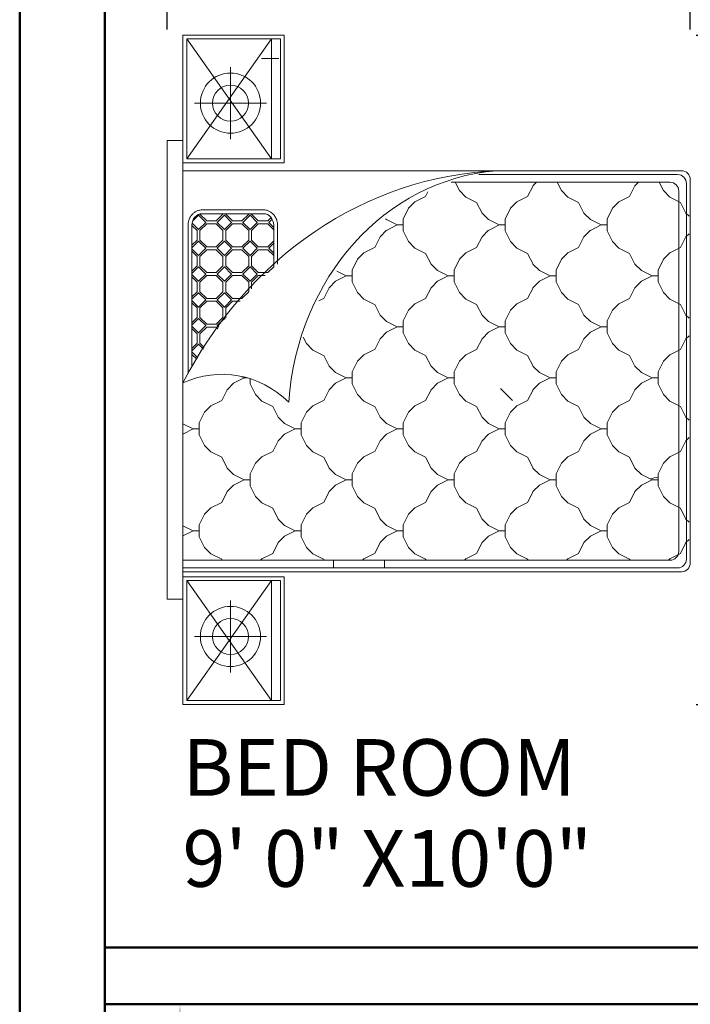
# Model space of a CAD drawing. Units: inches. Extents: x 2385 to 2740, y 1752 to 2305.
# Tile 8 of 15: x 2414 to 2485, y 2141 to 2245. Entities that reach past the tile are written whole.
import ezdxf

# ---------------------------------------------------------------- set-up
doc = ezdxf.new("R2010")
doc.units = ezdxf.units.IN
for name, color, linetype, lineweight in [('A-ANNO-DIMS', 2, 'Continuous', 18), ('A-AREA-IDEN', 7, 'Continuous', 25), ('A-FURN', 9, 'Continuous', 18), ('A-WALL', 7, 'Continuous', 50)]:
    doc.layers.add(name, color=color, linetype=linetype, lineweight=lineweight)
doc.styles.get("Standard").update_dxf_attribs({"font": 'arial.ttf'})
doc.dimstyles.new('Copy of ISO-25', dxfattribs={"dimtxt": 2.5, "dimasz": 2.5, "dimexe": 1.25, "dimexo": 0.625, "dimtad": 1, "dimdec": 1, "dimlunit": 4, "dimtxsty": 'Standard', "dimcen": 2.5, "dimadec": 0, "dimazin": 0, "dimtfac": 1, "dimtdec": 1, "dimtmove": 0, "dimatfit": 3, "dimfxl": 1, "dimarcsym": 0})

# ---------------------------------------------------------------- blocks, each defined once
blk = doc.blocks.new('A$C029D5C69')
for p, q in [((0.4164, 2.0693), (0.4164, 2.0066)), ((2.2315, 2.0693), (0.4164, 2.0693)), ((2.2315, 2.0066), (2.2315, 2.0693)), ((0, 1.606), (0, 2.0066)), ((0, 2.0066), (0.505, 2.0066)), ((0.0151, 1.6211), (0.0151, 1.9915)), ((0.0151, 1.9915), (0.4899, 1.9915)), ((0.4164, 2.0066), (2.2315, 2.0066)), ((0.4899, 1.9915), (0.4899, 1.6211)), ((0.505, 2.0066), (0.505, 1.606)), ((0.5252, 0.0351), (0.5252, 2.0066)), ((0.5403, 0.0502), (0.5403, 2.0066)), ((0.5706, 0.0805), (0.5706, 2.0066)), ((0.6869, 1.966), (0.6666, 2.0066)), ((0.7072, 2.0066), (0.6869, 1.966)), ((1.0902, 1.966), (1.0699, 2.0066)), ((1.1106, 2.0066), (1.0902, 1.966)), ((2.1114, 2.0087), (2.1114, 0.0351)), ((2.6479, 2.0066), (2.1429, 2.0066)), ((2.1429, 2.0066), (2.1429, 1.606)), ((2.6328, 1.9915), (2.158, 1.9915)), ((2.158, 1.9915), (2.158, 1.6211)), ((2.6328, 1.6211), (2.6328, 1.9915)), ((2.6479, 1.606), (2.6479, 2.0066)), ((0.2689, 1.9609), (0.2689, 1.6764)), ((0.6869, 1.9425), (0.6869, 1.966)), ((0.6869, 1.9425), (0.6869, 1.966)), ((1.0902, 1.9425), (1.0902, 1.966)), ((1.0902, 1.9425), (1.0902, 1.966)), ((1.8954, 1.9865), (1.3081, 1.9865)), ((1.8954, 1.9713), (1.3339, 1.9713)), ((1.3849, 1.9713), (1.3656, 1.952)), ((1.3945, 1.9713), (1.3714, 1.9483)), ((1.4249, 1.945), (1.3986, 1.9713)), ((1.4288, 1.9507), (1.4081, 1.9713)), ((1.4476, 1.9507), (1.4288, 1.9507)), ((1.4476, 1.9507), (1.4664, 1.9507)), ((1.487, 1.9713), (1.4664, 1.9507)), ((1.4966, 1.9713), (1.4703, 1.945)), ((1.527, 1.945), (1.5007, 1.9713)), ((1.5309, 1.9507), (1.5102, 1.9713)), ((1.5497, 1.9507), (1.5309, 1.9507)), ((1.5497, 1.9507), (1.5685, 1.9507)), ((1.5891, 1.9713), (1.5685, 1.9507)), ((1.5987, 1.9713), (1.5724, 1.945)), ((1.6291, 1.945), (1.6028, 1.9713)), ((1.633, 1.9507), (1.6123, 1.9713)), ((1.6518, 1.9507), (1.633, 1.9507)), ((1.6518, 1.9507), (1.6706, 1.9507)), ((1.6912, 1.9713), (1.6706, 1.9507)), ((1.7008, 1.9713), (1.6745, 1.945)), ((1.7312, 1.945), (1.7049, 1.9713)), ((1.7351, 1.9507), (1.7144, 1.9713)), ((1.7539, 1.9507), (1.7351, 1.9507)), ((1.7539, 1.9507), (1.7727, 1.9507)), ((1.7933, 1.9713), (1.7727, 1.9507)), ((1.8029, 1.9713), (1.7766, 1.945)), ((1.8333, 1.945), (1.807, 1.9713)), ((1.8372, 1.9507), (1.8165, 1.9713)), ((1.856, 1.9507), (1.8372, 1.9507)), ((1.856, 1.9507), (1.8748, 1.9507)), ((1.8954, 1.9713), (1.8748, 1.9507)), ((1.9043, 1.9707), (1.8787, 1.945)), ((1.9354, 1.945), (1.9114, 1.969)), ((2.379, 1.9609), (2.379, 1.6764)), ((0.621, 1.9213), (0.5955, 1.8958)), ((0.6634, 1.9425), (0.621, 1.9213)), ((0.6634, 1.9425), (0.621, 1.9213)), ((0.6869, 1.9425), (0.6634, 1.9425)), ((0.6869, 1.9425), (0.7104, 1.9425)), ((0.7528, 1.9213), (0.7104, 1.9425)), ((0.7528, 1.9213), (0.7104, 1.9425)), ((0.7783, 1.8958), (0.7528, 1.9213)), ((1.0243, 1.9213), (0.9988, 1.8958)), ((1.0668, 1.9425), (1.0244, 1.9213)), ((1.0668, 1.9425), (1.0244, 1.9213)), ((1.0902, 1.9425), (1.0668, 1.9425)), ((1.0902, 1.9425), (1.1137, 1.9425)), ((1.1561, 1.9213), (1.1137, 1.9425)), ((1.1561, 1.9213), (1.1137, 1.9425)), ((1.1816, 1.8958), (1.1561, 1.9213)), ((1.4249, 1.945), (1.4059, 1.926)), ((1.4288, 1.9394), (1.4116, 1.9222)), ((1.4288, 1.9393), (1.4476, 1.9393)), ((1.4664, 1.9393), (1.4476, 1.9393)), ((1.493, 1.9128), (1.4664, 1.9394)), ((1.4986, 1.9167), (1.4703, 1.945)), ((1.493, 1.8752), (1.493, 1.9128)), ((1.527, 1.945), (1.4986, 1.9167)), ((1.5309, 1.9394), (1.5043, 1.9128)), ((1.5043, 1.8752), (1.5043, 1.9128)), ((1.5309, 1.9393), (1.5497, 1.9393)), ((1.5685, 1.9393), (1.5497, 1.9393)), ((1.595, 1.9128), (1.5685, 1.9394)), ((1.6007, 1.9167), (1.5724, 1.945)), ((1.595, 1.8752), (1.595, 1.9128)), ((1.6291, 1.945), (1.6007, 1.9167)), ((1.633, 1.9394), (1.6064, 1.9128)), ((1.6064, 1.8752), (1.6064, 1.9128)), ((1.633, 1.9393), (1.6518, 1.9393)), ((1.6706, 1.9393), (1.6518, 1.9393)), ((1.6971, 1.9128), (1.6706, 1.9394)), ((1.7028, 1.9167), (1.6745, 1.945)), ((1.6971, 1.8752), (1.6971, 1.9128)), ((1.7312, 1.945), (1.7028, 1.9167)), ((1.7351, 1.9394), (1.7085, 1.9128)), ((1.7085, 1.8752), (1.7085, 1.9128)), ((1.7351, 1.9393), (1.7539, 1.9393)), ((1.7727, 1.9393), (1.7539, 1.9393)), ((1.7992, 1.9128), (1.7727, 1.9394)), ((1.8049, 1.9167), (1.7766, 1.945)), ((1.7992, 1.8752), (1.7992, 1.9128)), ((1.8333, 1.945), (1.8049, 1.9167)), ((1.8372, 1.9394), (1.8106, 1.9128)), ((1.8106, 1.8752), (1.8106, 1.9128)), ((1.8372, 1.9393), (1.856, 1.9393)), ((1.8748, 1.9393), (1.856, 1.9393)), ((1.9013, 1.9128), (1.8748, 1.9394)), ((1.907, 1.9167), (1.8787, 1.945)), ((1.9013, 1.8752), (1.9013, 1.9128)), ((1.9354, 1.945), (1.907, 1.9167)), ((1.9393, 1.9394), (1.9127, 1.9128)), ((1.9127, 1.8752), (1.9127, 1.9128)), ((1.9393, 1.9393), (1.9404, 1.9393)), ((1.9414, 1.688), (1.9414, 1.931)), ((1.9565, 1.688), (1.9565, 1.931)), ((0.5955, 1.8958), (0.5743, 1.8534)), ((0.7995, 1.8534), (0.7783, 1.8958)), ((0.9989, 1.8958), (0.9777, 1.8534)), ((1.2028, 1.8534), (1.1816, 1.8958)), ((1.493, 1.8752), (1.4867, 1.869)), ((1.4986, 1.8713), (1.4922, 1.8648)), ((1.527, 1.8429), (1.4986, 1.8713)), ((1.5309, 1.8486), (1.5043, 1.8752)), ((1.595, 1.8752), (1.5685, 1.8486)), ((1.6007, 1.8713), (1.5724, 1.8429)), ((1.6291, 1.8429), (1.6007, 1.8713)), ((1.633, 1.8486), (1.6064, 1.8752)), ((1.6971, 1.8752), (1.6706, 1.8486)), ((1.7028, 1.8713), (1.6745, 1.8429)), ((1.7312, 1.8429), (1.7028, 1.8713)), ((1.7351, 1.8486), (1.7085, 1.8752)), ((1.7992, 1.8752), (1.7727, 1.8486)), ((1.8049, 1.8713), (1.7766, 1.8429)), ((1.8333, 1.8429), (1.8049, 1.8713)), ((1.8372, 1.8486), (1.8106, 1.8752)), ((1.9013, 1.8752), (1.8748, 1.8486)), ((1.907, 1.8713), (1.8787, 1.8429)), ((1.9354, 1.8429), (1.907, 1.8713)), ((1.9393, 1.8486), (1.9127, 1.8752)), ((0.5743, 1.8534), (0.5706, 1.8515)), ((0.5743, 1.8534), (0.5706, 1.8515)), ((0.8419, 1.8322), (0.7995, 1.8534)), ((0.8419, 1.8322), (0.7995, 1.8534)), ((0.8674, 1.8067), (0.8419, 1.8322)), ((0.9352, 1.8322), (0.9097, 1.8067)), ((0.9777, 1.8534), (0.9353, 1.8322)), ((0.9777, 1.8534), (0.9353, 1.8322)), ((1.2452, 1.8322), (1.2028, 1.8534)), ((1.2452, 1.8322), (1.2028, 1.8534)), ((1.2707, 1.8067), (1.2452, 1.8322)), ((1.527, 1.8429), (1.5242, 1.8401)), ((1.5309, 1.8373), (1.5295, 1.8359)), ((1.5497, 1.8486), (1.5309, 1.8486)), ((1.5309, 1.8373), (1.5497, 1.8373)), ((1.5497, 1.8486), (1.5685, 1.8486)), ((1.5685, 1.8373), (1.5497, 1.8373)), ((1.595, 1.8107), (1.5685, 1.8373)), ((1.6007, 1.8146), (1.5724, 1.8429)), ((1.6291, 1.8429), (1.6007, 1.8146)), ((1.633, 1.8373), (1.6064, 1.8107)), ((1.6518, 1.8486), (1.633, 1.8486)), ((1.633, 1.8373), (1.6518, 1.8373)), ((1.6518, 1.8486), (1.6706, 1.8486)), ((1.6706, 1.8373), (1.6518, 1.8373)), ((1.6971, 1.8107), (1.6706, 1.8373)), ((1.7028, 1.8146), (1.6745, 1.8429)), ((1.7312, 1.8429), (1.7028, 1.8146)), ((1.7351, 1.8373), (1.7085, 1.8107)), ((1.7539, 1.8486), (1.7351, 1.8486)), ((1.7351, 1.8373), (1.7539, 1.8373)), ((1.7539, 1.8486), (1.7727, 1.8486)), ((1.7727, 1.8373), (1.7539, 1.8373)), ((1.7992, 1.8107), (1.7727, 1.8373)), ((1.8049, 1.8146), (1.7766, 1.8429)), ((1.8333, 1.8429), (1.8049, 1.8146)), ((1.8372, 1.8373), (1.8106, 1.8107)), ((1.856, 1.8486), (1.8372, 1.8486)), ((1.8372, 1.8373), (1.856, 1.8373)), ((1.856, 1.8486), (1.8748, 1.8486)), ((1.8748, 1.8373), (1.856, 1.8373)), ((1.9013, 1.8107), (1.8748, 1.8373)), ((1.907, 1.8146), (1.8787, 1.8429)), ((1.9354, 1.8429), (1.907, 1.8146)), ((1.9393, 1.8373), (1.9127, 1.8107)), ((1.9414, 1.8486), (1.9393, 1.8486)), ((1.9393, 1.8373), (1.9414, 1.8373)), ((0.1267, 1.8186), (0.4111, 1.8186)), ((0.8886, 1.7643), (0.8674, 1.8067)), ((0.9098, 1.8067), (0.8886, 1.7643)), ((1.2919, 1.7643), (1.2707, 1.8067)), ((1.595, 1.7806), (1.595, 1.8107)), ((1.6064, 1.7731), (1.6064, 1.8107)), ((1.6971, 1.7731), (1.6971, 1.8107)), ((1.7085, 1.7731), (1.7085, 1.8107)), ((1.7992, 1.7731), (1.7992, 1.8107)), ((1.8106, 1.7731), (1.8106, 1.8107)), ((1.9013, 1.7731), (1.9013, 1.8107)), ((1.9127, 1.7731), (1.9127, 1.8107)), ((2.2367, 1.8186), (2.5212, 1.8186)), ((0.8886, 1.7408), (0.8886, 1.7643)), ((1.2981, 1.7768), (1.2919, 1.7643)), ((1.2919, 1.7519), (1.2919, 1.7643)), ((1.633, 1.7465), (1.6064, 1.7731)), ((1.6971, 1.7731), (1.6706, 1.7465)), ((1.7028, 1.7692), (1.6745, 1.7408)), ((1.7312, 1.7408), (1.7028, 1.7692)), ((1.7351, 1.7465), (1.7085, 1.7731)), ((1.7992, 1.7731), (1.7727, 1.7465)), ((1.8049, 1.7692), (1.7766, 1.7408)), ((1.8333, 1.7408), (1.8049, 1.7692)), ((1.8372, 1.7465), (1.8106, 1.7731)), ((1.9013, 1.7731), (1.8748, 1.7465)), ((1.907, 1.7692), (1.8787, 1.7408)), ((1.9354, 1.7408), (1.907, 1.7692)), ((1.9393, 1.7465), (1.9127, 1.7731)), ((0.8227, 1.7196), (0.7972, 1.6941)), ((0.8651, 1.7408), (0.8227, 1.7196)), ((0.8651, 1.7408), (0.8227, 1.7196)), ((0.912, 1.7408), (0.8651, 1.7408)), ((0.9544, 1.7196), (0.912, 1.7408)), ((0.9544, 1.7196), (0.912, 1.7408)), ((0.98, 1.6941), (0.9545, 1.7196)), ((1.226, 1.7196), (1.2005, 1.6941)), ((1.2684, 1.7408), (1.226, 1.7196)), ((1.2684, 1.7408), (1.226, 1.7196)), ((1.2885, 1.7408), (1.2684, 1.7408)), ((1.6518, 1.7465), (1.633, 1.7465)), ((1.6443, 1.7352), (1.6518, 1.7352)), ((1.6518, 1.7465), (1.6706, 1.7465)), ((1.6706, 1.7352), (1.6518, 1.7352)), ((1.6971, 1.7086), (1.6706, 1.7352)), ((1.7028, 1.7125), (1.6745, 1.7408)), ((1.7312, 1.7408), (1.7028, 1.7125)), ((1.7351, 1.7352), (1.7085, 1.7086)), ((1.7539, 1.7465), (1.7351, 1.7465)), ((1.7351, 1.7352), (1.7539, 1.7352)), ((1.7539, 1.7465), (1.7727, 1.7465)), ((1.7727, 1.7352), (1.7539, 1.7352)), ((1.7992, 1.7086), (1.7727, 1.7352)), ((1.8049, 1.7125), (1.7766, 1.7408)), ((1.8333, 1.7408), (1.8049, 1.7125)), ((1.8372, 1.7352), (1.8106, 1.7086)), ((1.856, 1.7465), (1.8372, 1.7465)), ((1.8372, 1.7352), (1.856, 1.7352)), ((1.856, 1.7465), (1.8748, 1.7465)), ((1.8748, 1.7352), (1.856, 1.7352)), ((1.9013, 1.7086), (1.8748, 1.7352)), ((1.907, 1.7125), (1.8787, 1.7408)), ((1.9354, 1.7408), (1.907, 1.7125)), ((1.9393, 1.7352), (1.9127, 1.7086)), ((1.9414, 1.7465), (1.9393, 1.7465)), ((1.9393, 1.7352), (1.9414, 1.7352)), ((0.5766, 1.6941), (0.5706, 1.7002)), ((0.5978, 1.6517), (0.5766, 1.6941)), ((0.7972, 1.6941), (0.776, 1.6517)), ((1.0011, 1.6517), (0.9799, 1.6941)), ((1.2005, 1.6941), (1.1793, 1.6517)), ((1.6971, 1.682), (1.6971, 1.7086)), ((1.7085, 1.671), (1.7085, 1.7086)), ((1.7992, 1.671), (1.7992, 1.7086)), ((1.8106, 1.671), (1.8106, 1.7086)), ((1.9013, 1.671), (1.9013, 1.7086)), ((1.9127, 1.671), (1.9127, 1.7086)), ((2.5551, 1.6275), (2.5551, 1.696)), ((0.6402, 1.6305), (0.5978, 1.6517)), ((0.6402, 1.6305), (0.5978, 1.6517)), ((0.776, 1.6517), (0.7336, 1.6305)), ((0.776, 1.6517), (0.7336, 1.6305)), ((1.0435, 1.6305), (1.0011, 1.6517)), ((1.0435, 1.6305), (1.0011, 1.6517)), ((1.1793, 1.6517), (1.1369, 1.6305)), ((1.1793, 1.6517), (1.1369, 1.6305)), ((1.7318, 1.6477), (1.7085, 1.671)), ((1.8961, 1.6477), (1.7289, 1.6477)), ((1.7992, 1.671), (1.7759, 1.6477)), ((1.8049, 1.6671), (1.7855, 1.6477)), ((1.8244, 1.6477), (1.8049, 1.6671)), ((1.8339, 1.6477), (1.8106, 1.671)), ((1.9013, 1.671), (1.878, 1.6477)), ((1.907, 1.6671), (1.8876, 1.6477)), ((1.9202, 1.6539), (1.907, 1.6671)), ((1.926, 1.6577), (1.9127, 1.671)), ((0.505, 1.606), (0, 1.606)), ((0.4899, 1.6211), (0.0151, 1.6211)), ((0.6657, 1.605), (0.6402, 1.6305)), ((0.6869, 1.5626), (0.6657, 1.605)), ((0.7081, 1.605), (0.6869, 1.5626)), ((0.7336, 1.6305), (0.7081, 1.605)), ((1.0691, 1.605), (1.0436, 1.6305)), ((1.0902, 1.5626), (1.069, 1.605)), ((1.1114, 1.605), (1.0902, 1.5626)), ((1.1369, 1.6305), (1.1114, 1.605)), ((1.8961, 1.6325), (1.7422, 1.6325)), ((2.1429, 1.606), (2.6479, 1.606)), ((2.158, 1.6211), (2.6328, 1.6211)), ((0.6869, 1.5392), (0.6869, 1.5626)), ((0.6869, 1.5392), (0.6869, 1.5626)), ((1.0902, 1.5392), (1.0902, 1.5626)), ((1.0902, 1.5392), (1.0902, 1.5626)), ((0.6634, 1.5391), (0.621, 1.5179)), ((0.6634, 1.5391), (0.621, 1.5179)), ((0.6869, 1.5392), (0.6634, 1.5392)), ((0.6869, 1.5392), (0.7104, 1.5392)), ((0.7528, 1.5179), (0.7104, 1.5391)), ((0.7528, 1.5179), (0.7104, 1.5391)), ((1.0668, 1.5391), (1.0244, 1.5179)), ((1.0668, 1.5391), (1.0244, 1.5179)), ((1.0902, 1.5392), (1.0668, 1.5392)), ((1.0902, 1.5392), (1.1137, 1.5392)), ((1.1561, 1.5179), (1.1137, 1.5391)), ((1.1561, 1.5179), (1.1137, 1.5391)), ((1.4534, 1.5308), (1.4277, 1.5179)), ((1.4534, 1.5308), (1.4277, 1.5179)), ((0.5955, 1.4925), (0.5743, 1.4501)), ((0.621, 1.5179), (0.5955, 1.4924)), ((0.7783, 1.4924), (0.7528, 1.5179)), ((0.7995, 1.4501), (0.7783, 1.4925)), ((0.9989, 1.4925), (0.9777, 1.4501)), ((1.0243, 1.5179), (0.9988, 1.4924)), ((1.1816, 1.4924), (1.1561, 1.5179)), ((1.2028, 1.4501), (1.1816, 1.4925)), ((1.4022, 1.4925), (1.381, 1.4501)), ((1.4277, 1.5179), (1.4022, 1.4924)), ((0.5743, 1.45), (0.5706, 1.4481)), ((0.5743, 1.45), (0.5706, 1.4481)), ((0.8419, 1.4288), (0.7995, 1.45)), ((0.8419, 1.4288), (0.7995, 1.45)), ((0.9777, 1.45), (0.9353, 1.4288)), ((0.9777, 1.45), (0.9353, 1.4288)), ((1.2452, 1.4288), (1.2028, 1.45)), ((1.2452, 1.4288), (1.2028, 1.45)), ((1.381, 1.45), (1.3386, 1.4288)), ((1.381, 1.45), (1.3386, 1.4288)), ((1.6062, 1.4501), (1.5966, 1.4692)), ((1.6486, 1.4288), (1.6062, 1.45)), ((1.6486, 1.4288), (1.6062, 1.45)), ((0.5403, 1.4117), (0.5706, 1.4117)), ((0.8674, 1.4033), (0.8419, 1.4288)), ((0.8886, 1.361), (0.8674, 1.4034)), ((0.9098, 1.4034), (0.8886, 1.361)), ((0.9352, 1.4288), (0.9097, 1.4033)), ((1.2707, 1.4033), (1.2452, 1.4288)), ((1.2919, 1.361), (1.2707, 1.4034)), ((1.3131, 1.4034), (1.2919, 1.361)), ((1.3386, 1.4288), (1.3131, 1.4033)), ((1.6741, 1.4033), (1.6486, 1.4288)), ((1.6953, 1.361), (1.6741, 1.4034)), ((1.714, 1.3984), (1.6953, 1.361)), ((0.8651, 1.3374), (0.8227, 1.3162)), ((0.8651, 1.3374), (0.8227, 1.3162)), ((0.912, 1.3375), (0.8651, 1.3375)), ((0.8886, 1.3375), (0.8886, 1.3609)), ((0.9544, 1.3162), (0.912, 1.3374)), ((0.9544, 1.3162), (0.912, 1.3374)), ((1.2684, 1.3374), (1.226, 1.3162)), ((1.2684, 1.3374), (1.226, 1.3162)), ((1.3154, 1.3375), (1.2684, 1.3375)), ((1.2919, 1.3375), (1.2919, 1.3609)), ((1.3578, 1.3162), (1.3154, 1.3374)), ((1.3578, 1.3162), (1.3154, 1.3374)), ((1.6718, 1.3374), (1.6294, 1.3162)), ((1.6718, 1.3374), (1.6294, 1.3162)), ((1.7187, 1.3375), (1.6718, 1.3375)), ((1.6953, 1.3375), (1.6953, 1.3609)), ((1.7611, 1.3162), (1.7187, 1.3374)), ((1.7611, 1.3162), (1.7187, 1.3374)), ((0.5766, 1.2908), (0.5706, 1.2968)), ((0.5978, 1.2484), (0.5766, 1.2908)), ((0.7972, 1.2908), (0.776, 1.2484)), ((0.8227, 1.3163), (0.7972, 1.2908)), ((0.98, 1.2908), (0.9545, 1.3163)), ((1.0011, 1.2484), (0.9799, 1.2908)), ((1.2005, 1.2908), (1.1793, 1.2484)), ((1.226, 1.3163), (1.2005, 1.2908)), ((1.3833, 1.2908), (1.3578, 1.3163)), ((1.4045, 1.2484), (1.3833, 1.2908)), ((1.6039, 1.2908), (1.5827, 1.2484)), ((1.6294, 1.3163), (1.6039, 1.2908)), ((1.7867, 1.2908), (1.7611, 1.3163)), ((1.8078, 1.2484), (1.7866, 1.2908)), ((0.6402, 1.2271), (0.5978, 1.2483)), ((0.6402, 1.2271), (0.5978, 1.2483)), ((0.776, 1.2483), (0.7336, 1.2271)), ((0.776, 1.2483), (0.7336, 1.2271)), ((1.0435, 1.2271), (1.0011, 1.2483)), ((1.0435, 1.2271), (1.0011, 1.2483)), ((1.1793, 1.2483), (1.1369, 1.2271)), ((1.1793, 1.2483), (1.1369, 1.2271)), ((1.4469, 1.2271), (1.4045, 1.2483)), ((1.4469, 1.2271), (1.4045, 1.2483)), ((1.5827, 1.2483), (1.5403, 1.2271)), ((1.5827, 1.2483), (1.5403, 1.2271)), ((1.8502, 1.2271), (1.8078, 1.2483)), ((1.8502, 1.2271), (1.8078, 1.2483)), ((0.5403, 1.21), (0.5706, 1.21)), ((0.6657, 1.2017), (0.6402, 1.2272)), ((0.7336, 1.2272), (0.7081, 1.2017)), ((1.0691, 1.2017), (1.0436, 1.2272)), ((1.1369, 1.2272), (1.1114, 1.2017)), ((1.4724, 1.2017), (1.4469, 1.2272)), ((1.5403, 1.2272), (1.5148, 1.2017)), ((1.8758, 1.2017), (1.8503, 1.2272)), ((0.6869, 1.1593), (0.6657, 1.2017)), ((0.7081, 1.2017), (0.6869, 1.1593)), ((1.0902, 1.1593), (1.069, 1.2017)), ((1.1114, 1.2017), (1.0902, 1.1593)), ((1.4936, 1.1593), (1.4724, 1.2017)), ((1.5148, 1.2017), (1.4936, 1.1593)), ((1.8969, 1.1593), (1.8757, 1.2017)), ((1.9181, 1.2017), (1.8969, 1.1593)), ((1.9215, 1.2051), (1.9181, 1.2017)), ((0.6634, 1.1358), (0.621, 1.1146)), ((0.6634, 1.1358), (0.621, 1.1146)), ((0.6869, 1.1358), (0.6634, 1.1358)), ((0.6869, 1.1358), (0.6869, 1.1593)), ((0.6869, 1.1358), (0.6869, 1.1593)), ((0.6869, 1.1358), (0.7104, 1.1358)), ((0.7528, 1.1146), (0.7104, 1.1358)), ((0.7528, 1.1146), (0.7104, 1.1358)), ((1.0668, 1.1358), (1.0244, 1.1146)), ((1.0668, 1.1358), (1.0244, 1.1146)), ((1.0902, 1.1358), (1.0668, 1.1358)), ((1.0902, 1.1358), (1.0902, 1.1593)), ((1.0902, 1.1358), (1.0902, 1.1593)), ((1.0902, 1.1358), (1.1137, 1.1358)), ((1.1561, 1.1146), (1.1137, 1.1358)), ((1.1561, 1.1146), (1.1137, 1.1358)), ((1.4701, 1.1358), (1.4277, 1.1146)), ((1.4701, 1.1358), (1.4277, 1.1146)), ((1.4936, 1.1358), (1.4701, 1.1358)), ((1.4936, 1.1358), (1.4936, 1.1593)), ((1.4936, 1.1358), (1.4936, 1.1593)), ((1.4936, 1.1358), (1.5171, 1.1358)), ((1.5595, 1.1146), (1.5171, 1.1358)), ((1.5595, 1.1146), (1.5171, 1.1358)), ((1.8735, 1.1358), (1.8311, 1.1146)), ((1.8735, 1.1358), (1.8311, 1.1146)), ((1.8969, 1.1358), (1.8735, 1.1358)), ((1.8969, 1.1358), (1.8969, 1.1593)), ((1.8969, 1.1358), (1.8969, 1.1593)), ((1.8969, 1.1358), (1.9204, 1.1358)), ((1.9628, 1.1146), (1.9204, 1.1358)), ((1.9628, 1.1146), (1.9204, 1.1358)), ((0.621, 1.1146), (0.5955, 1.0891)), ((0.7783, 1.0891), (0.7528, 1.1146)), ((1.0243, 1.1146), (0.9988, 1.0891)), ((1.1816, 1.0891), (1.1561, 1.1146)), ((1.4277, 1.1146), (1.4022, 1.0891)), ((1.585, 1.0891), (1.5595, 1.1146)), ((1.831, 1.1146), (1.8055, 1.0891)), ((1.9883, 1.0891), (1.9628, 1.1146)), ((0.5955, 1.0891), (0.5743, 1.0467)), ((0.7995, 1.0467), (0.7783, 1.0891)), ((0.9989, 1.0891), (0.9777, 1.0467)), ((1.2028, 1.0467), (1.1816, 1.0891)), ((1.4022, 1.0891), (1.381, 1.0467)), ((1.6062, 1.0467), (1.585, 1.0891)), ((1.8056, 1.0891), (1.7844, 1.0467)), ((2.0095, 1.0467), (1.9883, 1.0891)), ((0.5743, 1.0467), (0.5706, 1.0448)), ((0.5743, 1.0467), (0.5706, 1.0448)), ((0.8419, 1.0255), (0.7995, 1.0467)), ((0.8419, 1.0255), (0.7995, 1.0467)), ((0.8674, 1), (0.8419, 1.0255)), ((0.9352, 1.0255), (0.9097, 1)), ((0.9777, 1.0467), (0.9353, 1.0255)), ((0.9777, 1.0467), (0.9353, 1.0255)), ((1.2452, 1.0255), (1.2028, 1.0467)), ((1.2452, 1.0255), (1.2028, 1.0467)), ((1.2707, 1), (1.2452, 1.0255)), ((1.3386, 1.0255), (1.3131, 1)), ((1.381, 1.0467), (1.3386, 1.0255)), ((1.381, 1.0467), (1.3386, 1.0255)), ((1.6486, 1.0255), (1.6062, 1.0467)), ((1.6486, 1.0255), (1.6062, 1.0467)), ((1.6741, 1), (1.6486, 1.0255)), ((1.7419, 1.0255), (1.7164, 1)), ((1.7844, 1.0467), (1.742, 1.0255)), ((1.7844, 1.0467), (1.742, 1.0255)), ((2.0276, 1.0376), (2.0095, 1.0467)), ((2.0276, 1.0376), (2.0095, 1.0467)), ((0.8886, 0.9576), (0.8674, 1)), ((0.9098, 1), (0.8886, 0.9576)), ((1.2919, 0.9576), (1.2707, 1)), ((1.3131, 1), (1.2919, 0.9576)), ((1.6953, 0.9576), (1.6741, 1)), ((1.7165, 1), (1.6953, 0.9576)), ((0.8886, 0.9341), (0.8886, 0.9576)), ((1.2919, 0.9341), (1.2919, 0.9576)), ((1.6953, 0.9341), (1.6953, 0.9576)), ((2.066, 0.9457), (2.066, 0.0805)), ((0.8227, 0.9129), (0.7972, 0.8874)), ((0.8651, 0.9341), (0.8227, 0.9129)), ((0.8651, 0.9341), (0.8227, 0.9129)), ((0.912, 0.9341), (0.8651, 0.9341)), ((0.9544, 0.9129), (0.912, 0.9341)), ((0.9544, 0.9129), (0.912, 0.9341)), ((0.98, 0.8874), (0.9545, 0.9129)), ((1.226, 0.9129), (1.2005, 0.8874)), ((1.2684, 0.9341), (1.226, 0.9129)), ((1.2684, 0.9341), (1.226, 0.9129)), ((1.3154, 0.9341), (1.2684, 0.9341)), ((1.3578, 0.9129), (1.3154, 0.9341)), ((1.3578, 0.9129), (1.3154, 0.9341)), ((1.3833, 0.8874), (1.3578, 0.9129)), ((1.6294, 0.9129), (1.6039, 0.8874)), ((1.6718, 0.9341), (1.6294, 0.9129)), ((1.6718, 0.9341), (1.6294, 0.9129)), ((1.7187, 0.9341), (1.6718, 0.9341)), ((1.7611, 0.9129), (1.7187, 0.9341)), ((1.7611, 0.9129), (1.7187, 0.9341)), ((1.7867, 0.8874), (1.7611, 0.9129)), ((2.0327, 0.9129), (2.0072, 0.8874)), ((2.066, 0.9295), (2.0327, 0.9129)), ((2.066, 0.9295), (2.0327, 0.9129)), ((0.5766, 0.8874), (0.5706, 0.8935)), ((0.5978, 0.845), (0.5766, 0.8874)), ((0.7972, 0.8874), (0.776, 0.845)), ((1.0011, 0.845), (0.9799, 0.8874)), ((1.2005, 0.8874), (1.1793, 0.845)), ((1.4045, 0.845), (1.3833, 0.8874)), ((1.6039, 0.8874), (1.5827, 0.845)), ((1.8078, 0.845), (1.7866, 0.8874)), ((2.0072, 0.8874), (1.986, 0.845)), ((0.6402, 0.8238), (0.5978, 0.845)), ((0.6402, 0.8238), (0.5978, 0.845)), ((0.6657, 0.7983), (0.6402, 0.8238)), ((0.7336, 0.8238), (0.7081, 0.7983)), ((0.776, 0.845), (0.7336, 0.8238)), ((0.776, 0.845), (0.7336, 0.8238)), ((1.0435, 0.8238), (1.0011, 0.845)), ((1.0435, 0.8238), (1.0011, 0.845)), ((1.0691, 0.7983), (1.0436, 0.8238)), ((1.1369, 0.8238), (1.1114, 0.7983)), ((1.1793, 0.845), (1.1369, 0.8238)), ((1.1793, 0.845), (1.1369, 0.8238)), ((1.4469, 0.8238), (1.4045, 0.845)), ((1.4469, 0.8238), (1.4045, 0.845)), ((1.4724, 0.7983), (1.4469, 0.8238)), ((1.5403, 0.8238), (1.5148, 0.7983)), ((1.5827, 0.845), (1.5403, 0.8238)), ((1.5827, 0.845), (1.5403, 0.8238)), ((1.8502, 0.8238), (1.8078, 0.845)), ((1.8502, 0.8238), (1.8078, 0.845)), ((1.8758, 0.7983), (1.8503, 0.8238)), ((1.9436, 0.8238), (1.9181, 0.7983)), ((1.986, 0.845), (1.9436, 0.8238)), ((1.986, 0.845), (1.9436, 0.8238)), ((2.0962, 0.8369), (2.0962, 0.0502)), ((0.6869, 0.7559), (0.6657, 0.7983)), ((0.7081, 0.7983), (0.6869, 0.7559)), ((1.0902, 0.7559), (1.069, 0.7983)), ((1.1114, 0.7983), (1.0902, 0.7559)), ((1.4936, 0.7559), (1.4724, 0.7983)), ((1.5148, 0.7983), (1.4936, 0.7559)), ((1.8969, 0.7559), (1.8757, 0.7983)), ((1.9181, 0.7983), (1.8969, 0.7559)), ((0.6869, 0.7325), (0.6869, 0.7559)), ((0.6869, 0.7325), (0.6869, 0.7559)), ((1.0902, 0.7325), (1.0902, 0.7559)), ((1.0902, 0.7325), (1.0902, 0.7559)), ((1.2024, 0.7028), (1.2503, 0.7507)), ((1.4936, 0.7325), (1.4936, 0.7559)), ((1.4936, 0.7325), (1.4936, 0.7559)), ((1.8969, 0.7325), (1.8969, 0.7559)), ((1.8969, 0.7325), (1.8969, 0.7559)), ((0.621, 0.7113), (0.5955, 0.6858)), ((0.6634, 0.7324), (0.621, 0.7112)), ((0.6634, 0.7324), (0.621, 0.7112)), ((0.6869, 0.7325), (0.6634, 0.7325)), ((0.6869, 0.7325), (0.7104, 0.7325)), ((0.7528, 0.7112), (0.7104, 0.7324)), ((0.7528, 0.7112), (0.7104, 0.7324)), ((0.7783, 0.6858), (0.7528, 0.7113)), ((1.0243, 0.7113), (0.9988, 0.6858)), ((1.0668, 0.7324), (1.0244, 0.7112)), ((1.0668, 0.7324), (1.0244, 0.7112)), ((1.0902, 0.7325), (1.0668, 0.7325)), ((1.0902, 0.7325), (1.1137, 0.7325)), ((1.1561, 0.7112), (1.1137, 0.7324)), ((1.1561, 0.7112), (1.1137, 0.7324)), ((1.1816, 0.6858), (1.1561, 0.7113)), ((1.4277, 0.7113), (1.4022, 0.6858)), ((1.4701, 0.7324), (1.4277, 0.7112)), ((1.4701, 0.7324), (1.4277, 0.7112)), ((1.4936, 0.7325), (1.4701, 0.7325)), ((1.4936, 0.7325), (1.5171, 0.7325)), ((1.5595, 0.7112), (1.5171, 0.7324)), ((1.5595, 0.7112), (1.5171, 0.7324)), ((1.585, 0.6858), (1.5595, 0.7113)), ((1.831, 0.7113), (1.8055, 0.6858)), ((1.8735, 0.7324), (1.8311, 0.7112)), ((1.8735, 0.7324), (1.8311, 0.7112)), ((1.8969, 0.7325), (1.8735, 0.7325)), ((1.8969, 0.7325), (1.9204, 0.7325)), ((1.9628, 0.7112), (1.9204, 0.7324)), ((1.9628, 0.7112), (1.9204, 0.7324)), ((1.9883, 0.6858), (1.9628, 0.7113)), ((0.5955, 0.6858), (0.5743, 0.6434)), ((0.7995, 0.6434), (0.7783, 0.6858)), ((0.9989, 0.6858), (0.9777, 0.6434)), ((1.2028, 0.6434), (1.1816, 0.6858)), ((1.4022, 0.6858), (1.381, 0.6434)), ((1.6062, 0.6434), (1.585, 0.6858)), ((1.8056, 0.6858), (1.7844, 0.6434)), ((2.0095, 0.6434), (1.9883, 0.6858)), ((0.5743, 0.6433), (0.5706, 0.6414)), ((0.5743, 0.6433), (0.5706, 0.6414)), ((0.8419, 0.6221), (0.7995, 0.6433)), ((0.8419, 0.6221), (0.7995, 0.6433)), ((0.9777, 0.6433), (0.9353, 0.6221)), ((0.9777, 0.6433), (0.9353, 0.6221)), ((1.2452, 0.6221), (1.2028, 0.6433)), ((1.2452, 0.6221), (1.2028, 0.6433)), ((1.381, 0.6433), (1.3386, 0.6221)), ((1.381, 0.6433), (1.3386, 0.6221)), ((1.6486, 0.6221), (1.6062, 0.6433)), ((1.6486, 0.6221), (1.6062, 0.6433)), ((1.7844, 0.6433), (1.742, 0.6221)), ((1.7844, 0.6433), (1.742, 0.6221)), ((2.0519, 0.6221), (2.0095, 0.6433)), ((2.0519, 0.6221), (2.0095, 0.6433)), ((0.8674, 0.5967), (0.8419, 0.6222)), ((0.8886, 0.5543), (0.8674, 0.5967)), ((0.9098, 0.5967), (0.8886, 0.5543)), ((0.9352, 0.6222), (0.9097, 0.5967)), ((1.2707, 0.5967), (1.2452, 0.6222)), ((1.2919, 0.5543), (1.2707, 0.5967)), ((1.3131, 0.5967), (1.2919, 0.5543)), ((1.3386, 0.6222), (1.3131, 0.5967)), ((1.6741, 0.5967), (1.6486, 0.6222)), ((1.6953, 0.5543), (1.6741, 0.5967)), ((1.7165, 0.5967), (1.6953, 0.5543)), ((1.7419, 0.6222), (1.7164, 0.5967)), ((2.066, 0.6081), (2.0519, 0.6222)), ((0.8886, 0.5308), (0.8886, 0.5543)), ((1.2919, 0.5308), (1.2919, 0.5543)), ((1.6953, 0.5308), (1.6953, 0.5543)), ((0.8227, 0.5096), (0.7972, 0.4841)), ((0.8651, 0.5308), (0.8227, 0.5096)), ((0.8651, 0.5308), (0.8227, 0.5096)), ((0.912, 0.5308), (0.8651, 0.5308)), ((0.9544, 0.5096), (0.912, 0.5308)), ((0.9544, 0.5096), (0.912, 0.5308)), ((0.98, 0.4841), (0.9545, 0.5096)), ((1.226, 0.5096), (1.2005, 0.4841)), ((1.2684, 0.5308), (1.226, 0.5096)), ((1.2684, 0.5308), (1.226, 0.5096)), ((1.3154, 0.5308), (1.2684, 0.5308)), ((1.3578, 0.5096), (1.3154, 0.5308)), ((1.3578, 0.5096), (1.3154, 0.5308)), ((1.3833, 0.4841), (1.3578, 0.5096)), ((1.6294, 0.5096), (1.6039, 0.4841)), ((1.6718, 0.5308), (1.6294, 0.5096)), ((1.6718, 0.5308), (1.6294, 0.5096)), ((1.7187, 0.5308), (1.6718, 0.5308)), ((1.7611, 0.5096), (1.7187, 0.5308)), ((1.7611, 0.5096), (1.7187, 0.5308)), ((1.7867, 0.4841), (1.7611, 0.5096)), ((2.0327, 0.5096), (2.0072, 0.4841)), ((2.066, 0.5262), (2.0327, 0.5096)), ((2.066, 0.5262), (2.0327, 0.5096)), ((0.5766, 0.4841), (0.5706, 0.4901)), ((0.5978, 0.4417), (0.5766, 0.4841)), ((0.7972, 0.4841), (0.776, 0.4417)), ((1.0011, 0.4417), (0.9799, 0.4841)), ((1.2005, 0.4841), (1.1793, 0.4417)), ((1.4045, 0.4417), (1.3833, 0.4841)), ((1.6039, 0.4841), (1.5827, 0.4417)), ((1.8078, 0.4417), (1.7866, 0.4841)), ((2.0072, 0.4841), (1.986, 0.4417)), ((0.6402, 0.4205), (0.5978, 0.4417)), ((0.6402, 0.4205), (0.5978, 0.4417)), ((0.776, 0.4417), (0.7336, 0.4205)), ((0.776, 0.4417), (0.7336, 0.4205)), ((1.0435, 0.4205), (1.0011, 0.4417)), ((1.0435, 0.4205), (1.0011, 0.4417)), ((1.1793, 0.4417), (1.1369, 0.4205)), ((1.1793, 0.4417), (1.1369, 0.4205)), ((1.4469, 0.4205), (1.4045, 0.4417)), ((1.4469, 0.4205), (1.4045, 0.4417)), ((1.5827, 0.4417), (1.5403, 0.4205)), ((1.5827, 0.4417), (1.5403, 0.4205)), ((1.8502, 0.4205), (1.8078, 0.4417)), ((1.8502, 0.4205), (1.8078, 0.4417)), ((1.986, 0.4417), (1.9436, 0.4205)), ((1.986, 0.4417), (1.9436, 0.4205)), ((0.6657, 0.395), (0.6402, 0.4205)), ((0.6869, 0.3526), (0.6657, 0.395)), ((0.7081, 0.395), (0.6869, 0.3526)), ((0.7336, 0.4205), (0.7081, 0.395)), ((1.0691, 0.395), (1.0436, 0.4205)), ((1.0902, 0.3526), (1.069, 0.395)), ((1.1114, 0.395), (1.0902, 0.3526)), ((1.1369, 0.4205), (1.1114, 0.395)), ((1.4724, 0.395), (1.4469, 0.4205)), ((1.4936, 0.3526), (1.4724, 0.395)), ((1.5148, 0.395), (1.4936, 0.3526)), ((1.5403, 0.4205), (1.5148, 0.395)), ((1.8758, 0.395), (1.8503, 0.4205)), ((1.8969, 0.3526), (1.8757, 0.395)), ((1.9181, 0.395), (1.8969, 0.3526)), ((1.9436, 0.4205), (1.9181, 0.395)), ((0.6869, 0.3291), (0.6869, 0.3526)), ((0.6869, 0.3291), (0.6869, 0.3526)), ((1.0902, 0.3291), (1.0902, 0.3526)), ((1.0902, 0.3291), (1.0902, 0.3526)), ((1.4936, 0.3291), (1.4936, 0.3526)), ((1.4936, 0.3291), (1.4936, 0.3526)), ((1.8969, 0.3291), (1.8969, 0.3526)), ((1.8969, 0.3291), (1.8969, 0.3526)), ((0.6634, 0.3291), (0.621, 0.3079)), ((0.6634, 0.3291), (0.621, 0.3079)), ((0.6869, 0.3291), (0.6634, 0.3291)), ((0.6869, 0.3291), (0.7104, 0.3291)), ((0.7528, 0.3079), (0.7104, 0.3291)), ((0.7528, 0.3079), (0.7104, 0.3291)), ((1.0668, 0.3291), (1.0244, 0.3079)), ((1.0668, 0.3291), (1.0244, 0.3079)), ((1.0902, 0.3291), (1.0668, 0.3291)), ((1.0902, 0.3291), (1.1137, 0.3291)), ((1.1561, 0.3079), (1.1137, 0.3291)), ((1.1561, 0.3079), (1.1137, 0.3291)), ((1.4701, 0.3291), (1.4277, 0.3079)), ((1.4701, 0.3291), (1.4277, 0.3079)), ((1.4936, 0.3291), (1.4701, 0.3291)), ((1.4936, 0.3291), (1.5171, 0.3291)), ((1.5595, 0.3079), (1.5171, 0.3291)), ((1.5595, 0.3079), (1.5171, 0.3291)), ((1.8735, 0.3291), (1.8311, 0.3079)), ((1.8735, 0.3291), (1.8311, 0.3079)), ((1.8969, 0.3291), (1.8735, 0.3291)), ((1.8969, 0.3291), (1.9204, 0.3291)), ((1.9628, 0.3079), (1.9204, 0.3291)), ((1.9628, 0.3079), (1.9204, 0.3291)), ((0.5955, 0.2824), (0.5743, 0.24)), ((0.621, 0.3079), (0.5955, 0.2824)), ((0.7783, 0.2824), (0.7528, 0.3079)), ((0.7995, 0.24), (0.7783, 0.2824)), ((0.9989, 0.2824), (0.9777, 0.24)), ((1.0243, 0.3079), (0.9988, 0.2824)), ((1.1816, 0.2824), (1.1561, 0.3079)), ((1.2028, 0.24), (1.1816, 0.2824)), ((1.4022, 0.2824), (1.381, 0.24)), ((1.4277, 0.3079), (1.4022, 0.2824)), ((1.585, 0.2824), (1.5595, 0.3079)), ((1.6062, 0.24), (1.585, 0.2824)), ((1.8056, 0.2824), (1.7844, 0.24)), ((1.831, 0.3079), (1.8055, 0.2824)), ((1.9883, 0.2824), (1.9628, 0.3079)), ((2.0095, 0.24), (1.9883, 0.2824)), ((0.5743, 0.24), (0.5706, 0.2381)), ((0.5743, 0.24), (0.5706, 0.2381)), ((0.8419, 0.2188), (0.7995, 0.24)), ((0.8419, 0.2188), (0.7995, 0.24)), ((0.9777, 0.24), (0.9353, 0.2188)), ((0.9777, 0.24), (0.9353, 0.2188)), ((1.2452, 0.2188), (1.2028, 0.24)), ((1.2452, 0.2188), (1.2028, 0.24)), ((1.381, 0.24), (1.3386, 0.2188)), ((1.381, 0.24), (1.3386, 0.2188)), ((1.6486, 0.2188), (1.6062, 0.24)), ((1.6486, 0.2188), (1.6062, 0.24)), ((1.7844, 0.24), (1.742, 0.2188)), ((1.7844, 0.24), (1.742, 0.2188)), ((2.0519, 0.2188), (2.0095, 0.24)), ((2.0519, 0.2188), (2.0095, 0.24)), ((0.8674, 0.1933), (0.8419, 0.2188)), ((0.9352, 0.2188), (0.9097, 0.1933)), ((1.2707, 0.1933), (1.2452, 0.2188)), ((1.3386, 0.2188), (1.3131, 0.1933)), ((1.6741, 0.1933), (1.6486, 0.2188)), ((1.7419, 0.2188), (1.7164, 0.1933)), ((2.066, 0.2047), (2.0519, 0.2188)), ((0.8886, 0.1509), (0.8674, 0.1933)), ((0.9098, 0.1933), (0.8886, 0.1509)), ((1.2919, 0.1509), (1.2707, 0.1933)), ((1.3131, 0.1933), (1.2919, 0.1509)), ((1.6953, 0.1509), (1.6741, 0.1933)), ((1.7165, 0.1933), (1.6953, 0.1509)), ((0.8651, 0.1274), (0.8227, 0.1062)), ((0.8651, 0.1274), (0.8227, 0.1062)), ((0.912, 0.1275), (0.8651, 0.1275)), ((0.8886, 0.1275), (0.8886, 0.1509)), ((0.9544, 0.1062), (0.912, 0.1274)), ((0.9544, 0.1062), (0.912, 0.1274)), ((1.2684, 0.1274), (1.226, 0.1062)), ((1.2684, 0.1274), (1.226, 0.1062)), ((1.3154, 0.1275), (1.2684, 0.1275)), ((1.2919, 0.1275), (1.2919, 0.1509)), ((1.3578, 0.1062), (1.3154, 0.1274)), ((1.3578, 0.1062), (1.3154, 0.1274)), ((1.6718, 0.1274), (1.6294, 0.1062)), ((1.6718, 0.1274), (1.6294, 0.1062)), ((1.7187, 0.1275), (1.6718, 0.1275)), ((1.6953, 0.1275), (1.6953, 0.1509)), ((1.7611, 0.1062), (1.7187, 0.1274)), ((1.7611, 0.1062), (1.7187, 0.1274)), ((2.066, 0.1228), (2.0327, 0.1062)), ((2.066, 0.1228), (2.0327, 0.1062)), ((0.5766, 0.0807), (0.5706, 0.0868)), ((0.5978, 0.0384), (0.5766, 0.0808)), ((0.7972, 0.0808), (0.776, 0.0384)), ((0.8227, 0.1062), (0.7972, 0.0807)), ((0.98, 0.0807), (0.9545, 0.1062)), ((1.0011, 0.0384), (0.9799, 0.0808)), ((1.2005, 0.0808), (1.1793, 0.0384)), ((1.226, 0.1062), (1.2005, 0.0807)), ((1.3833, 0.0807), (1.3578, 0.1062)), ((1.4045, 0.0384), (1.3833, 0.0808)), ((1.6039, 0.0808), (1.5827, 0.0384)), ((1.6294, 0.1062), (1.6039, 0.0807)), ((1.7867, 0.0807), (1.7611, 0.1062)), ((1.8078, 0.0384), (1.7866, 0.0808)), ((2.0072, 0.0808), (1.986, 0.0384)), ((2.0327, 0.1062), (2.0072, 0.0807)), ((2.0309, 0.0454), (0.6056, 0.0454)), ((2.0763, 0), (0.5603, 0)), ((2.0612, 0.0151), (0.5754, 0.0151)), ((0.6402, 0.0171), (0.5978, 0.0383)), ((0.6402, 0.0171), (0.5978, 0.0383)), ((0.6523, 0.005), (0.6402, 0.0171)), ((0.7336, 0.0171), (0.7215, 0.005)), ((0.776, 0.0383), (0.7336, 0.0171)), ((0.776, 0.0383), (0.7336, 0.0171)), ((1.0435, 0.0171), (1.0011, 0.0383)), ((1.0435, 0.0171), (1.0011, 0.0383)), ((1.0557, 0.005), (1.0436, 0.0171)), ((1.1369, 0.0171), (1.1248, 0.005)), ((1.1793, 0.0383), (1.1369, 0.0171)), ((1.1793, 0.0383), (1.1369, 0.0171)), ((1.4469, 0.0171), (1.4045, 0.0383)), ((1.4469, 0.0171), (1.4045, 0.0383)), ((1.459, 0.005), (1.4469, 0.0171)), ((1.5403, 0.0171), (1.5282, 0.005)), ((1.5827, 0.0383), (1.5403, 0.0171)), ((1.5827, 0.0383), (1.5403, 0.0171)), ((1.8502, 0.0171), (1.8078, 0.0383)), ((1.8502, 0.0171), (1.8078, 0.0383)), ((1.8623, 0.005), (1.8503, 0.0171)), ((1.9436, 0.0171), (1.9315, 0.005)), ((1.986, 0.0383), (1.9436, 0.0171)), ((1.986, 0.0383), (1.9436, 0.0171))]:
    blk.add_line(p, q)
at = {"ltscale": 0.005}
for p, q in [((0.4899, 1.6568), (0.0151, 1.9915)), ((0.0151, 1.6568), (0.4899, 1.9915)), ((2.6328, 1.6568), (2.158, 1.9915)), ((2.158, 1.6568), (2.6328, 1.9915)), ((0.0151, 1.6568), (0.4899, 1.6568)), ((2.6328, 1.6568), (2.158, 1.6568))]:
    blk.add_line(p, q, dxfattribs=at)
for centre, radius in [((0.2689, 1.8186), 0.1191), ((2.379, 1.8186), 0.1191), ((0.2689, 1.8186), 0.0711), ((2.379, 1.8186), 0.0711)]:
    blk.add_circle(centre, radius)
for centre, radius, start, end in [((0.2843, 0.0157), 0.6251, 10.2961, 13.2684), ((0.6056, 0.0805), 0.0351, 180, 270), ((2.0309, 0.0805), 0.0351, 270, 0), ((0.5754, 0.0502), 0.0351, 180, 270), ((2.0612, 0.0502), 0.0351, 270, 0), ((0.5603, 0.0351), 0.0351, 180, 270), ((2.0763, 0.0351), 0.0351, 270, 0)]:
    blk.add_arc(centre, radius, start, end)
for centre, major_axis, ratio, start_param, end_param in [((0.8506, 1.8527), (-0.4556, 0), 0.89, 2.430919, 3.53111), ((0.3667, 0.6698), (1.7398, 0.1668), 0.88072, -0.045073, 0.941433), ((1.8961, 1.931), (-0.0453, 0), 0.89, 3.141593, 4.712389), ((1.8961, 1.688), (-0.0453, 0), 0.89, 1.570796, 3.141593), ((1.0874, 0.6748), (1.021, 0.1213), 0.889348, -0.031673, 1.359628)]:
    blk.add_ellipse(centre, major_axis=major_axis, ratio=ratio, start_param=start_param, end_param=end_param)
for points, knots in [([(1.9565, 1.931), (1.9565, 1.9336), (1.9563, 1.9362), (1.9553, 1.9428), (1.9543, 1.9467), (1.9512, 1.9541), (1.9493, 1.9577), (1.9446, 1.9643), (1.942, 1.9674), (1.936, 1.9729), (1.9327, 1.9753), (1.9257, 1.9795), (1.922, 1.9813), (1.9142, 1.9841), (1.9102, 1.9851), (1.9028, 1.9862), (1.8995, 1.9865), (1.8961, 1.9865)], [3.141593, 3.141593, 3.141593, 3.141593, 3.277614, 3.277614, 3.488082, 3.488082, 3.698551, 3.698551, 3.909019, 3.909019, 4.119488, 4.119488, 4.329956, 4.329956, 4.540424, 4.540424, 4.712389, 4.712389, 4.712389, 4.712389]), ([(1.8961, 1.6325), (1.899, 1.6325), (1.9019, 1.6327), (1.9101, 1.6338), (1.9153, 1.6352), (1.9253, 1.6392), (1.93, 1.6418), (1.9385, 1.6481), (1.9423, 1.6519), (1.9481, 1.6594), (1.9503, 1.663), (1.9537, 1.6707), (1.955, 1.6747), (1.9563, 1.6818), (1.9565, 1.6849), (1.9565, 1.688)], [1.570796, 1.570796, 1.570796, 1.570796, 1.718836, 1.718836, 1.993452, 1.993452, 2.268068, 2.268068, 2.542684, 2.542684, 2.761386, 2.761386, 2.980087, 2.980087, 3.141593, 3.141593, 3.141593, 3.141593])]:
    blk.add_open_spline(points, degree=3, knots=knots)
blk = doc.blocks.new('*D12')
at = {"layer": 'A-ANNO-DIMS', "color": 0, "lineweight": -2, "transparency": 16777216}
for p, q in [((2423.87, 2140.97), (2432.46, 2140.97)), ((2431.21, 2138.47), (2431.21, 1927.47)), ((2423.87, 1924.97), (2432.46, 1924.97))]:
    blk.add_line(p, q, dxfattribs=at)
at = {"layer": 'A-ANNO-DIMS', "color": 0, "transparency": 16777216}
for points in [[(2430.79, 2138.47), (2431.63, 2138.47), (2431.21, 2140.97)], [(2430.79, 1927.47), (2431.63, 1927.47), (2431.21, 1924.97)]]:
    blk.add_solid(points, dxfattribs=at)
at = {"layer": 'Defpoints', "color": 0, "transparency": 16777216}
for p in [(2423.25, 2140.97), (2423.25, 1924.97), (2431.21, 1924.97)]:
    blk.add_point(p, dxfattribs=at)
at = {"layer": 'A-ANNO-DIMS', "color": 0, "transparency": 16777216, "insert": (2429.31, 2032.97), "char_height": 2.5, "attachment_point": 5, "rotation": 90}
blk.add_mtext("18'", dxfattribs=at)
blk = doc.blocks.new('*D26')
at = {"layer": 'A-ANNO-DIMS', "color": 0, "lineweight": -2, "transparency": 16777216}
for p, q in [((2485.89, 2243.62), (2497.15, 2243.62)), ((2495.9, 2175.23), (2495.9, 2241.12)), ((2485.89, 2172.73), (2497.15, 2172.73))]:
    blk.add_line(p, q, dxfattribs=at)
at = {"layer": 'A-ANNO-DIMS', "color": 0, "transparency": 16777216}
for points in [[(2495.48, 2241.12), (2496.31, 2241.12), (2495.9, 2243.62)], [(2495.48, 2175.23), (2496.31, 2175.23), (2495.9, 2172.73)]]:
    blk.add_solid(points, dxfattribs=at)
at = {"layer": 'Defpoints', "color": 0, "transparency": 16777216}
for p in [(2485.26, 2243.62), (2495.9, 2243.62), (2485.26, 2172.73)]:
    blk.add_point(p, dxfattribs=at)
at = {"layer": 'A-ANNO-DIMS', "color": 0, "transparency": 16777216, "insert": (2493.99, 2208.17), "char_height": 2.5, "attachment_point": 5, "rotation": 90}
blk.add_mtext('BED 5\'-11" TYP.', dxfattribs=at)
blk = doc.blocks.new('*D27')
at = {"layer": 'A-ANNO-DIMS', "color": 0, "lineweight": -2, "transparency": 16777216}
for p, q in [((2429.86, 2244.24), (2429.86, 2255.5)), ((2485.26, 2244.24), (2485.26, 2255.5)), ((2482.76, 2254.25), (2432.36, 2254.25))]:
    blk.add_line(p, q, dxfattribs=at)
at = {"layer": 'A-ANNO-DIMS', "color": 0, "transparency": 16777216}
for points in [[(2432.36, 2254.67), (2432.36, 2253.84), (2429.86, 2254.25)], [(2482.76, 2254.67), (2482.76, 2253.84), (2485.26, 2254.25)]]:
    blk.add_solid(points, dxfattribs=at)
at = {"layer": 'Defpoints', "color": 0, "transparency": 16777216}
for p in [(2429.86, 2254.25), (2429.86, 2243.62), (2485.26, 2243.62)]:
    blk.add_point(p, dxfattribs=at)
at = {"layer": 'A-ANNO-DIMS', "color": 0, "transparency": 16777216, "insert": (2457.56, 2256.17), "char_height": 2.5, "attachment_point": 5}
blk.add_mtext('4\'-7 1/2" TYP.', dxfattribs=at)

msp = doc.modelspace()

# ---------------------------------------------------------------- linework, layer by layer
at = {"layer": 'A-WALL'}
for p, q in [((2414.25, 1924.97), (2414.25, 2266.97)), ((2423.25, 2266.97), (2423.25, 2146.97)), ((2423.25, 2146.97), (2423.25, 2140.97)), ((2423.25, 2140.97), (2423.25, 2146.97)), ((2423.25, 2146.97), (2495.25, 2146.97)), ((2495.25, 2140.97), (2423.25, 2140.97)), ((2423.25, 2140.97), (2423.25, 1924.97))]:
    msp.add_line(p, q, dxfattribs=at)

# ---------------------------------------------------------------- block references
at = {"layer": 'A-FURN', "xscale": 26.77336660145066, "yscale": 26.77336660145066, "zscale": 26.77336660145066, "rotation": 90}
msp.add_blockref('A$C029D5C69', (2485.26, 2172.73), dxfattribs=at)

# ---------------------------------------------------------------- texts
at = {"layer": 'A-AREA-IDEN'}
for s, p in [('BED ROOM', (2431.49, 2163.06)), ('9\' 0" X10\'0"', (2431.49, 2153.42))]:
    msp.add_text(s, height=6, dxfattribs=at).set_placement(p)

# ---------------------------------------------------------------- dimensions: what is measured, and where the dimension line sits
at = {"layer": 'A-ANNO-DIMS'}
for base, p1, p2, angle, text, picture, middle in [((2429.86, 2254.25), (2485.26, 2243.62), (2429.86, 2243.62), 180, '<> TYP.', '*D27', (2457.56, 2256.17)), ((2495.9, 2243.62), (2485.26, 2172.73), (2485.26, 2243.62), 90, 'BED <> TYP.', '*D26', (2493.99, 2208.17))]:
    dim = msp.add_linear_dim(base=base, p1=p1, p2=p2, angle=angle, text=text, dimstyle='Copy of ISO-25', override={"dimdec": 1, "dimlfac": 1, "dimrnd": 0, "dimzin": 1, "dimdsep": 46, "dimlunit": 4, "dimfrac": 2}, dxfattribs=at)
    dim.commit()
    dim.dimension.update_dxf_attribs({"geometry": picture, "text_midpoint": middle})
dim = msp.add_linear_dim(base=(2431.21, 1924.97), p1=(2423.25, 2140.97), p2=(2423.25, 1924.97), angle=90, dimstyle='Copy of ISO-25', override={"dimclrd": 0, "dimclre": 0, "dimclrt": 0}, dxfattribs=at)
dim.commit()
dim.dimension.update_dxf_attribs({"geometry": '*D12', "text_midpoint": (2429.31, 2032.97)})

doc.saveas('drawing.dxf')
